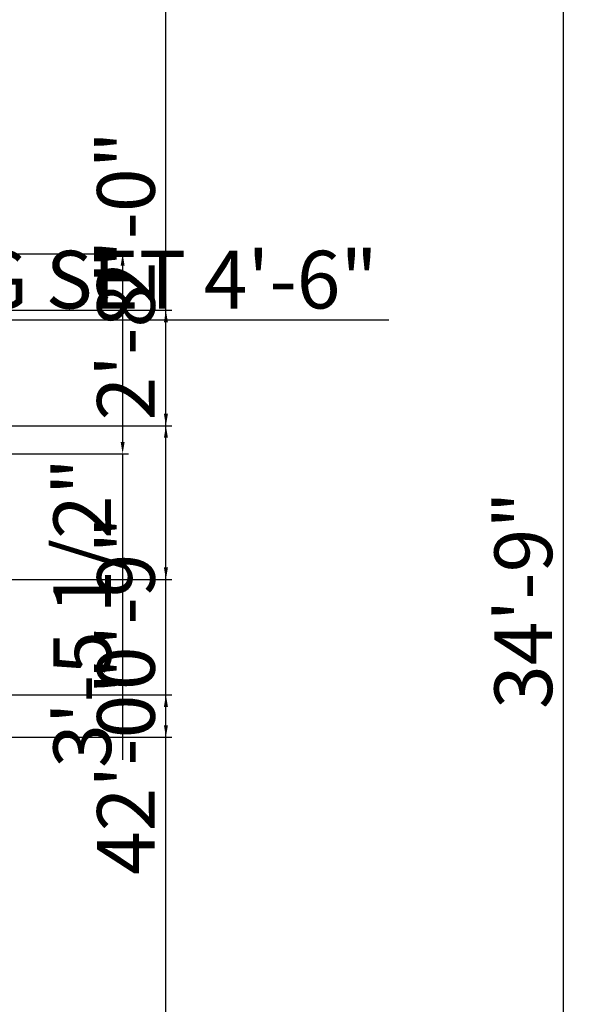
# Model space of a CAD drawing. Units: inches. Extents: x 1810 to 2254, y 313 to 1026.
# Tile 6 of 7: x 2139 to 2254, y 559 to 764. Entities that reach past the tile are written whole.
import ezdxf

# ---------------------------------------------------------------- set-up
doc = ezdxf.new("R2010")
doc.units = ezdxf.units.IN
doc.layers.add('A-ANNO-DIMS', color=2, linetype='Continuous', lineweight=18)
doc.styles.get("Standard").update_dxf_attribs({"font": 'arial.ttf'})
doc.dimstyles.new('ISO-25', dxfattribs={"dimtxt": 12, "dimasz": 2.5, "dimexe": 1.25, "dimexo": 0.625, "dimtad": 1, "dimdec": 1, "dimlunit": 4, "dimtxsty": 'Standard', "dimcen": 2.5, "dimadec": 0, "dimazin": 0, "dimtfac": 1, "dimtdec": 1, "dimtmove": 0, "dimatfit": 3, "dimfxl": 1, "dimarcsym": 0})

# ---------------------------------------------------------------- blocks, each defined once
blk = doc.blocks.new('*D23')
at = {"layer": 'A-ANNO-DIMS', "color": 0, "lineweight": -2, "transparency": 16777216}
for p, q in [((2130.99, 851.61), (2253.63, 851.61)), ((2252.38, 849.11), (2252.38, 437.11)), ((2130.99, 434.61), (2253.63, 434.61))]:
    blk.add_line(p, q, dxfattribs=at)
at = {"layer": 'A-ANNO-DIMS', "color": 0, "transparency": 16777216}
for points in [[(2251.96, 849.11), (2252.8, 849.11), (2252.38, 851.61)], [(2251.96, 437.11), (2252.8, 437.11), (2252.38, 434.61)]]:
    blk.add_solid(points, dxfattribs=at)
at = {"layer": 'Defpoints', "color": 0, "transparency": 16777216}
for p in [(2130.36, 851.61), (2130.36, 434.61), (2252.38, 434.61)]:
    blk.add_point(p, dxfattribs=at)
at = {"layer": 'A-ANNO-DIMS', "color": 0, "transparency": 16777216, "insert": (2245.62, 643.11), "char_height": 12, "attachment_point": 5, "rotation": 90}
blk.add_mtext('34\'-9"', dxfattribs=at)
blk = doc.blocks.new('*D46')
at = {"layer": 'A-ANNO-DIMS', "color": 0, "lineweight": -2, "transparency": 16777216}
for p, q in [((2026.69, 693.91), (2026.69, 702.6)), ((2080.48, 693.91), (2080.48, 702.6)), ((2029.19, 701.35), (2077.98, 701.35)), ((2080.48, 701.35), (2216.12, 701.35))]:
    blk.add_line(p, q, dxfattribs=at)
at = {"layer": 'A-ANNO-DIMS', "color": 0, "transparency": 16777216}
for points in [[(2029.19, 701.77), (2029.19, 700.93), (2026.69, 701.35)], [(2077.98, 701.77), (2077.98, 700.93), (2080.48, 701.35)]]:
    blk.add_solid(points, dxfattribs=at)
at = {"layer": 'Defpoints', "color": 0, "transparency": 16777216}
for p in [(2080.48, 701.35), (2026.69, 693.28), (2080.48, 693.28)]:
    blk.add_point(p, dxfattribs=at)
at = {"layer": 'A-ANNO-DIMS', "color": 0, "transparency": 16777216, "insert": (2149.55, 708.18), "char_height": 12, "attachment_point": 5}
blk.add_mtext('DINING SET 4\'-6"', dxfattribs=at)
blk = doc.blocks.new('*D50')
at = {"layer": 'A-ANNO-DIMS', "color": 0, "lineweight": -2, "transparency": 16777216}
for p, q in [((2139.99, 860.61), (2171.01, 860.61)), ((2169.76, 359.11), (2169.76, 858.11)), ((2139.99, 356.61), (2171.01, 356.61))]:
    blk.add_line(p, q, dxfattribs=at)
at = {"layer": 'A-ANNO-DIMS', "color": 0, "transparency": 16777216}
for points in [[(2169.35, 858.11), (2170.18, 858.11), (2169.76, 860.61)], [(2169.35, 359.11), (2170.18, 359.11), (2169.76, 356.61)]]:
    blk.add_solid(points, dxfattribs=at)
at = {"layer": 'Defpoints', "color": 0, "transparency": 16777216}
for p in [(2139.36, 860.61), (2169.76, 860.61), (2139.36, 356.61)]:
    blk.add_point(p, dxfattribs=at)
at = {"layer": 'A-ANNO-DIMS', "color": 0, "transparency": 16777216, "insert": (2163.01, 608.61), "char_height": 12, "attachment_point": 5, "rotation": 90}
blk.add_mtext('42\'-0"', dxfattribs=at)
blk = doc.blocks.new('*D54')
at = {"layer": 'A-ANNO-DIMS', "color": 0, "lineweight": -2, "transparency": 16777216}
for p, q in [((2130.99, 715.11), (2162.01, 715.11)), ((2160.76, 712.61), (2160.76, 676.02)), ((2130.99, 673.52), (2162.01, 673.52)), ((2160.76, 673.52), (2160.76, 609.92))]:
    blk.add_line(p, q, dxfattribs=at)
at = {"layer": 'A-ANNO-DIMS', "color": 0, "transparency": 16777216}
for points in [[(2160.35, 712.61), (2161.18, 712.61), (2160.76, 715.11)], [(2160.35, 676.02), (2161.18, 676.02), (2160.76, 673.52)]]:
    blk.add_solid(points, dxfattribs=at)
at = {"layer": 'Defpoints', "color": 0, "transparency": 16777216}
for p in [(2130.36, 715.11), (2130.36, 673.52), (2160.76, 673.52)]:
    blk.add_point(p, dxfattribs=at)
at = {"layer": 'A-ANNO-DIMS', "color": 0, "transparency": 16777216, "insert": (2153.93, 640.47), "char_height": 12, "attachment_point": 5, "rotation": 90}
blk.add_mtext('3\'-5 1/2"', dxfattribs=at)
blk = doc.blocks.new('*D57')
at = {"layer": 'A-ANNO-DIMS', "color": 0, "lineweight": -2, "transparency": 16777216}
for p, q in [((2104.86, 718.99), (2104.86, 323.71)), ((2130.36, 718.99), (2130.36, 323.71)), ((2107.36, 324.96), (2127.86, 324.96)), ((2130.36, 324.96), (2194.18, 324.96))]:
    blk.add_line(p, q, dxfattribs=at)
at = {"layer": 'A-ANNO-DIMS', "color": 0, "transparency": 16777216}
for points in [[(2107.36, 325.38), (2107.36, 324.55), (2104.86, 324.96)], [(2127.86, 325.38), (2127.86, 324.55), (2130.36, 324.96)]]:
    blk.add_solid(points, dxfattribs=at)
at = {"layer": 'Defpoints', "color": 0, "transparency": 16777216}
for p in [(2104.86, 719.61), (2130.36, 719.61), (2130.36, 324.96)]:
    blk.add_point(p, dxfattribs=at)
at = {"layer": 'A-ANNO-DIMS', "color": 0, "transparency": 16777216, "insert": (2163.52, 331.79), "char_height": 12, "attachment_point": 5}
blk.add_mtext('2\'-1 1/2"', dxfattribs=at)
blk = doc.blocks.new('*D61')
at = {"layer": 'A-ANNO-DIMS', "color": 0, "lineweight": -2, "transparency": 16777216}
for p, q in [((2106.36, 559.74), (2106.36, 892.26)), ((2108.86, 891.01), (2127.86, 891.01)), ((2130.36, 559.74), (2130.36, 892.26)), ((2130.36, 891.01), (2166.22, 891.01))]:
    blk.add_line(p, q, dxfattribs=at)
at = {"layer": 'A-ANNO-DIMS', "color": 0, "transparency": 16777216}
for points in [[(2108.86, 891.43), (2108.86, 890.6), (2106.36, 891.01)], [(2127.86, 891.43), (2127.86, 890.6), (2130.36, 891.01)]]:
    blk.add_solid(points, dxfattribs=at)
at = {"layer": 'Defpoints', "color": 0, "transparency": 16777216}
for p in [(2130.36, 891.01), (2106.36, 559.11), (2130.36, 559.11)]:
    blk.add_point(p, dxfattribs=at)
at = {"layer": 'A-ANNO-DIMS', "color": 0, "transparency": 16777216, "insert": (2149.54, 897.76), "char_height": 12, "attachment_point": 5}
blk.add_mtext('2\'-0"', dxfattribs=at)
blk = doc.blocks.new('*D62')
at = {"layer": 'A-ANNO-DIMS', "color": 0, "lineweight": -2, "transparency": 16777216}
for p, q in [((2169.76, 703.36), (2169.76, 739.21)), ((1973.49, 703.36), (2171.01, 703.36)), ((2169.76, 681.86), (2169.76, 700.86)), ((1973.49, 679.36), (2171.01, 679.36))]:
    blk.add_line(p, q, dxfattribs=at)
at = {"layer": 'A-ANNO-DIMS', "color": 0, "transparency": 16777216}
for points in [[(2169.35, 700.86), (2170.18, 700.86), (2169.76, 703.36)], [(2169.35, 681.86), (2170.18, 681.86), (2169.76, 679.36)]]:
    blk.add_solid(points, dxfattribs=at)
at = {"layer": 'Defpoints', "color": 0, "transparency": 16777216}
for p in [(1972.86, 703.36), (2169.76, 703.36), (1972.86, 679.36)]:
    blk.add_point(p, dxfattribs=at)
at = {"layer": 'A-ANNO-DIMS', "color": 0, "transparency": 16777216, "insert": (2163.01, 722.54), "char_height": 12, "attachment_point": 5, "rotation": 90}
blk.add_mtext('2\'-0"', dxfattribs=at)
blk = doc.blocks.new('*D63')
at = {"layer": 'A-ANNO-DIMS', "color": 0, "lineweight": -2, "transparency": 16777216}
for p, q in [((2169.76, 679.36), (2169.76, 715.21)), ((1973.49, 679.36), (2171.01, 679.36)), ((2169.76, 649.92), (2169.76, 676.86)), ((1973.49, 647.42), (2171.01, 647.42))]:
    blk.add_line(p, q, dxfattribs=at)
at = {"layer": 'A-ANNO-DIMS', "color": 0, "transparency": 16777216}
for points in [[(2169.35, 676.86), (2170.18, 676.86), (2169.76, 679.36)], [(2169.35, 649.92), (2170.18, 649.92), (2169.76, 647.42)]]:
    blk.add_solid(points, dxfattribs=at)
at = {"layer": 'Defpoints', "color": 0, "transparency": 16777216}
for p in [(1972.86, 679.36), (2169.76, 679.36), (1972.86, 647.42)]:
    blk.add_point(p, dxfattribs=at)
at = {"layer": 'A-ANNO-DIMS', "color": 0, "transparency": 16777216, "insert": (2163.01, 698.54), "char_height": 12, "attachment_point": 5, "rotation": 90}
blk.add_mtext('2\'-8"', dxfattribs=at)
blk = doc.blocks.new('*D64')
at = {"layer": 'A-ANNO-DIMS', "color": 0, "lineweight": -2, "transparency": 16777216}
for p, q in [((2169.76, 623.42), (2169.76, 659.07)), ((1973.49, 623.42), (2171.01, 623.42)), ((2169.76, 617.11), (2169.76, 620.92)), ((1973.49, 614.61), (2171.01, 614.61))]:
    blk.add_line(p, q, dxfattribs=at)
at = {"layer": 'A-ANNO-DIMS', "color": 0, "transparency": 16777216}
for points in [[(2169.35, 620.92), (2170.18, 620.92), (2169.76, 623.42)], [(2169.35, 617.11), (2170.18, 617.11), (2169.76, 614.61)]]:
    blk.add_solid(points, dxfattribs=at)
at = {"layer": 'Defpoints', "color": 0, "transparency": 16777216}
for p in [(1972.86, 623.42), (2169.76, 623.42), (1972.86, 614.61)]:
    blk.add_point(p, dxfattribs=at)
at = {"layer": 'A-ANNO-DIMS', "color": 0, "transparency": 16777216, "insert": (2163.01, 642.49), "char_height": 12, "attachment_point": 5, "rotation": 90}
blk.add_mtext('0\'-9"', dxfattribs=at)

msp = doc.modelspace()

# ---------------------------------------------------------------- dimensions: what is measured, and where the dimension line sits
at = {"layer": 'A-ANNO-DIMS'}
for base, p1, p2, picture, middle in [((2130.36, 891.01), (2106.36, 559.11), (2130.36, 559.11), '*D61', (2149.54, 897.76)), ((2130.36, 324.96), (2104.86, 719.61), (2130.36, 719.61), '*D57', (2163.52, 331.79))]:
    dim = msp.add_linear_dim(base=base, p1=p1, p2=p2, dimstyle='ISO-25', override={"dimdec": 1, "dimlfac": 1, "dimrnd": 0, "dimzin": 1, "dimdsep": 46, "dimlunit": 4, "dimfrac": 2}, dxfattribs=at)
    dim.commit()
    dim.dimension.update_dxf_attribs({"geometry": picture, "text_midpoint": middle})
for base, p1, p2, angle, override, picture, middle in [((2169.76, 860.61), (2139.36, 356.61), (2139.36, 860.61), 90, {"dimdec": 1, "dimlfac": 1, "dimrnd": 0, "dimzin": 1, "dimdsep": 46, "dimlunit": 4, "dimfrac": 2}, '*D50', (2163.01, 608.61)), ((2252.38, 434.61), (2130.36, 851.61), (2130.36, 434.61), 90, {"dimclrd": 0, "dimclre": 0, "dimclrt": 0}, '*D23', (2245.62, 643.11)), ((2169.76, 703.36), (1972.86, 679.36), (1972.86, 703.36), 90, {"dimdec": 1, "dimlfac": 1, "dimrnd": 0, "dimzin": 1, "dimdsep": 46, "dimlunit": 4, "dimfrac": 2}, '*D62', (2163.01, 722.54)), ((2169.76, 679.36), (1972.86, 647.42), (1972.86, 679.36), 90, {"dimdec": 1, "dimlfac": 1, "dimrnd": 0, "dimzin": 1, "dimdsep": 46, "dimlunit": 4, "dimfrac": 2}, '*D63', (2163.01, 698.54)), ((2160.76, 673.52), (2130.36, 715.11), (2130.36, 673.52), 270, {"dimdec": 1, "dimlfac": 1, "dimrnd": 0, "dimzin": 1, "dimdsep": 46, "dimlunit": 4, "dimfrac": 2}, '*D54', (2153.93, 640.47)), ((2169.76, 623.42), (1972.86, 614.61), (1972.86, 623.42), 90, {"dimdec": 1, "dimlfac": 1, "dimrnd": 0, "dimzin": 1, "dimdsep": 46, "dimlunit": 4, "dimfrac": 2}, '*D64', (2163.01, 642.49))]:
    dim = msp.add_linear_dim(base=base, p1=p1, p2=p2, angle=angle, dimstyle='ISO-25', override=override, dxfattribs=at)
    dim.commit()
    dim.dimension.update_dxf_attribs({"geometry": picture, "text_midpoint": middle})
dim = msp.add_linear_dim(base=(2080.48, 701.35), p1=(2026.69, 693.28), p2=(2080.48, 693.28), text='DINING SET <>', dimstyle='ISO-25', override={"dimdec": 1, "dimlfac": 1, "dimrnd": 0, "dimzin": 1, "dimdsep": 46, "dimlunit": 4, "dimfrac": 2}, dxfattribs=at)
dim.commit()
dim.dimension.update_dxf_attribs({"geometry": '*D46', "text_midpoint": (2149.55, 708.18)})

doc.saveas('drawing.dxf')
